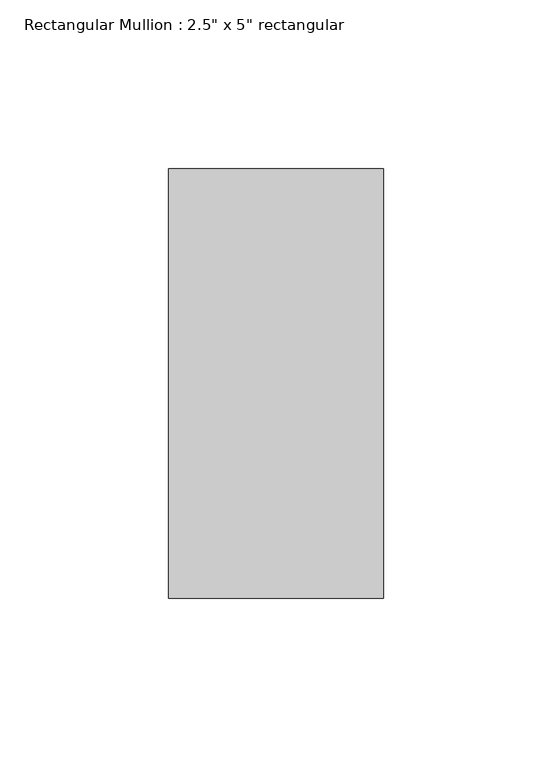
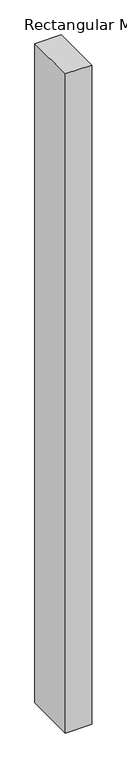
"""IFC4 building model written with IfcOpenShell, lengths in millimetres: member geometry."""

from ifc_helpers import new_model, si_unit, frame, origin, place, context, project, spatial, polyline, outline, extrude, source, transform, mapped, element, save


def member_c1cae106(model_context):
    return source(origin(), model_context, "Body", "SweptSolid", [
        extrude(outline(polyline([(0.0, 63.5), (0.0, -63.5), (-63.5, -63.5), (-63.5, 63.5), (0.0, 63.5)])), frame((0.0, 0.0, -1675.2875727), z_axis=(0.0, 0.0, 1.0), x_axis=(1.0, 0.0, 0.0)), (0.0, 0.0, 1.0), 1675.2875727),
    ])


if __name__ == "__main__":
    model = new_model("IFC4")
    model_context = context("Model", 3, world=origin())
    ifc_project = project(units=[si_unit("LENGTHUNIT", "METRE", prefix="MILLI")], contexts=[model_context])
    site = spatial("IfcSite", under=ifc_project)
    building = spatial("IfcBuilding", under=site)
    placement = place(None, origin())
    member_shape = member_c1cae106(model_context)
    element("IfcMember", 1, ObjectType="Rectangular Mullion : 2.5\" x 5\" rectangular", at=placement, inside=building, context=model_context, shape_type="MappedRepresentation", body=[
        mapped(member_shape, transform((0.0, 0.0, 0.0), x_axis=(1.0, 0.0, 0.0), y_axis=(0.0, 1.0, 0.0), z_axis=(0.0, 0.0, 1.0))),
    ])
    save(model, "model.ifc")

# Revit data of these elements
# Type "Rectangular Mullion : 2.5\" x 5\" rectangular"
#   built-in parameter 1007304 = 0.416667 (stored number, unit not read)
#   built-in parameter 1007301 = 0.104167 (stored number, unit not read)
#   built-in parameter 1007300 = 0.104167 (stored number, unit not read)
# Element 1 (IfcMember, "Rectangular Mullion : 2.5\" x 5\" rectangular")
#   Materials on its faces: "Aluminum"
# Materials
#   "Aluminum": class "Metal", colour RGB 247 247 247, transparency 0, Description = "Aluminum 6061", Cost = 0
